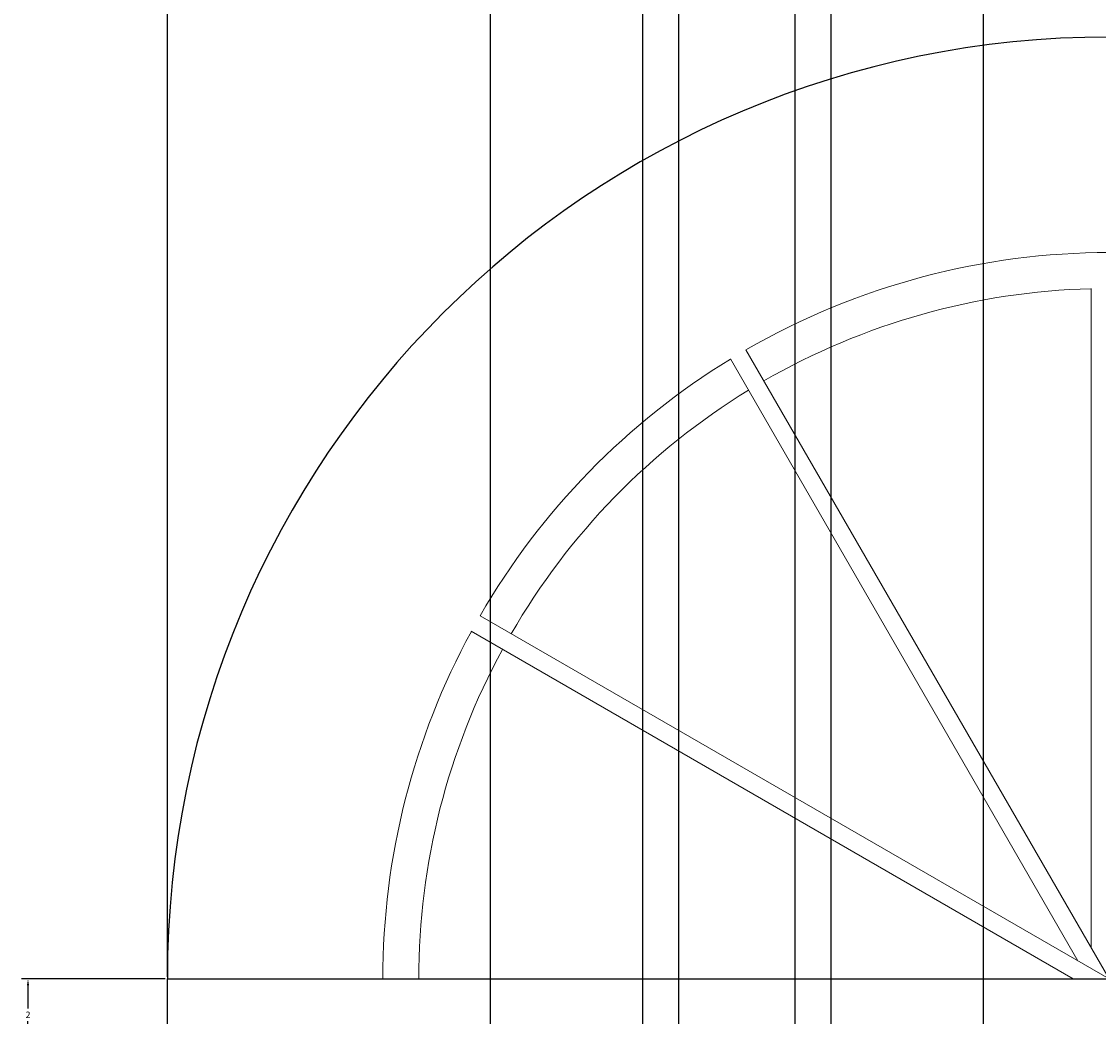
# Model space of a CAD drawing. Units: inches. Extents: x 12532.3 to 12594.9, y 6967.5 to 7063.
# Tile 6 of 9: x 12532.4 to 12562.4, y 7019.9 to 7047.6. Entities that reach past the tile are written whole.
import ezdxf

# ---------------------------------------------------------------- set-up
doc = ezdxf.new("R2010")
doc.units = ezdxf.units.IN
doc.header["$MEASUREMENT"] = 0
doc.header["$PDMODE"] = 98
for name, color, linetype, lineweight in [('A-ANNO-DIMS', 2, 'Continuous', 18), ('A-DOOR', 4, 'Continuous', 25), ('A-GLAZ', 3, 'Continuous', 18)]:
    doc.layers.add(name, color=color, linetype=linetype, lineweight=lineweight)
doc.styles.get("Standard").update_dxf_attribs({"font": 'arial.ttf'})
doc.dimstyles.get("Standard").update_dxf_attribs({"dimtxt": 0.18, "dimasz": 0.18, "dimexe": 0.18, "dimexo": 0.0625, "dimgap": 0.09, "dimtad": 0, "dimtih": 1, "dimtoh": 1, "dimdec": 4, "dimzin": 0, "dimdsep": 46, "dimtxsty": 'Standard', "dimcen": 0.09, "dimadec": 0, "dimazin": 0, "dimtfac": 1, "dimtdec": 4, "dimtofl": 0, "dimtmove": 0, "dimatfit": 3, "dimfxl": 1, "dimtolj": 1, "dimtzin": 0, "dimarcsym": 0})

# ---------------------------------------------------------------- blocks, each defined once
blk = doc.blocks.new('*D31')
at = {"layer": 'A-ANNO-DIMS', "color": 0, "lineweight": -2, "transparency": 16777216}
for p, q in [((12536.45, 7020.991), (12536.45, 7051.211)), ((12588.894, 7020.991), (12588.894, 7051.211)), ((12536.63, 7051.031), (12562.279, 7051.031)), ((12588.714, 7051.031), (12563.065, 7051.031))]:
    blk.add_line(p, q, dxfattribs=at)
at = {"layer": 'A-ANNO-DIMS', "color": 0, "transparency": 16777216}
for points in [[(12536.63, 7051.061), (12536.63, 7051.001), (12536.45, 7051.031)], [(12588.714, 7051.061), (12588.714, 7051.001), (12588.894, 7051.031)]]:
    blk.add_solid(points, dxfattribs=at)
at = {"layer": 'Defpoints', "color": 0, "transparency": 16777216}
for p in [(12588.894, 7051.031), (12536.45, 7020.929), (12588.894, 7020.929)]:
    blk.add_point(p, dxfattribs=at)
at = {"layer": 'A-ANNO-DIMS', "color": 0, "transparency": 16777216, "insert": (12562.672, 7051.031), "char_height": 0.18, "attachment_point": 5}
blk.add_mtext('\\A1;52.44', dxfattribs=at)
blk = doc.blocks.new('*D45')
at = {"layer": 'A-ANNO-DIMS', "color": 0, "lineweight": -2, "transparency": 16777216}
for p, q in [((12536.388, 7020.929), (12532.39, 7020.929)), ((12532.57, 7020.749), (12532.57, 7020.109)), ((12532.57, 7019.109), (12532.57, 7019.748)), ((12542.388, 7018.929), (12532.39, 7018.929))]:
    blk.add_line(p, q, dxfattribs=at)
at = {"layer": 'A-ANNO-DIMS', "color": 0, "transparency": 16777216}
for points in [[(12532.54, 7020.749), (12532.6, 7020.749), (12532.57, 7020.929)], [(12532.54, 7019.109), (12532.6, 7019.109), (12532.57, 7018.929)]]:
    blk.add_solid(points, dxfattribs=at)
at = {"layer": 'Defpoints', "color": 0, "transparency": 16777216}
for p in [(12532.57, 7020.929), (12536.45, 7020.929), (12542.45, 7018.929)]:
    blk.add_point(p, dxfattribs=at)
at = {"layer": 'A-ANNO-DIMS', "color": 0, "transparency": 16777216, "insert": (12532.57, 7019.929), "char_height": 0.18, "attachment_point": 5}
blk.add_mtext('\\A1;2', dxfattribs=at)
blk = doc.blocks.new('*D46')
at = {"layer": 'A-ANNO-DIMS', "color": 0, "lineweight": -2, "transparency": 16777216}
for p, q in [((12545.45, 7015.991), (12545.45, 7051.211)), ((12549.691, 7015.991), (12549.691, 7051.211)), ((12545.63, 7051.031), (12547.191, 7051.031)), ((12549.511, 7051.031), (12547.95, 7051.031))]:
    blk.add_line(p, q, dxfattribs=at)
at = {"layer": 'A-ANNO-DIMS', "color": 0, "transparency": 16777216}
for points in [[(12545.63, 7051.061), (12545.63, 7051.001), (12545.45, 7051.031)], [(12549.511, 7051.061), (12549.511, 7051.001), (12549.691, 7051.031)]]:
    blk.add_solid(points, dxfattribs=at)
at = {"layer": 'Defpoints', "color": 0, "transparency": 16777216}
for p in [(12549.691, 7051.031), (12545.45, 7015.929), (12549.691, 7015.929)]:
    blk.add_point(p, dxfattribs=at)
at = {"layer": 'A-ANNO-DIMS', "color": 0, "transparency": 16777216, "insert": (12547.57, 7051.031), "char_height": 0.18, "attachment_point": 5}
blk.add_mtext('\\A1;4.241', dxfattribs=at)
blk = doc.blocks.new('*D47')
at = {"layer": 'A-ANNO-DIMS', "color": 0, "lineweight": -2, "transparency": 16777216}
for p, q in [((12549.691, 7015.991), (12549.691, 7051.211)), ((12550.691, 7015.991), (12550.691, 7051.211)), ((12549.871, 7051.031), (12550.068, 7051.031)), ((12550.511, 7051.031), (12550.314, 7051.031))]:
    blk.add_line(p, q, dxfattribs=at)
at = {"layer": 'A-ANNO-DIMS', "color": 0, "transparency": 16777216}
for points in [[(12549.871, 7051.061), (12549.871, 7051.001), (12549.691, 7051.031)], [(12550.511, 7051.061), (12550.511, 7051.001), (12550.691, 7051.031)]]:
    blk.add_solid(points, dxfattribs=at)
at = {"layer": 'Defpoints', "color": 0, "transparency": 16777216}
for p in [(12550.691, 7051.031), (12549.691, 7015.929), (12550.691, 7015.929)]:
    blk.add_point(p, dxfattribs=at)
at = {"layer": 'A-ANNO-DIMS', "color": 0, "transparency": 16777216, "insert": (12550.191, 7051.031), "char_height": 0.18, "attachment_point": 5}
blk.add_mtext('\\A1;1', dxfattribs=at)
blk = doc.blocks.new('*D48')
at = {"layer": 'A-ANNO-DIMS', "color": 0, "lineweight": -2, "transparency": 16777216}
for p, q in [((12550.691, 7015.991), (12550.691, 7051.211)), ((12553.931, 7015.991), (12553.931, 7051.211)), ((12550.871, 7051.031), (12551.988, 7051.031)), ((12553.751, 7051.031), (12552.634, 7051.031))]:
    blk.add_line(p, q, dxfattribs=at)
at = {"layer": 'A-ANNO-DIMS', "color": 0, "transparency": 16777216}
for points in [[(12550.871, 7051.061), (12550.871, 7051.001), (12550.691, 7051.031)], [(12553.751, 7051.061), (12553.751, 7051.001), (12553.931, 7051.031)]]:
    blk.add_solid(points, dxfattribs=at)
at = {"layer": 'Defpoints', "color": 0, "transparency": 16777216}
for p in [(12553.931, 7051.031), (12550.691, 7015.929), (12553.931, 7015.929)]:
    blk.add_point(p, dxfattribs=at)
at = {"layer": 'A-ANNO-DIMS', "color": 0, "transparency": 16777216, "insert": (12552.311, 7051.031), "char_height": 0.18, "attachment_point": 5}
blk.add_mtext('\\A1;3.24', dxfattribs=at)
blk = doc.blocks.new('*D49')
at = {"layer": 'A-ANNO-DIMS', "color": 0, "lineweight": -2, "transparency": 16777216}
for p, q in [((12553.931, 7015.991), (12553.931, 7051.211)), ((12554.931, 7015.991), (12554.931, 7051.211)), ((12554.111, 7051.031), (12554.308, 7051.031)), ((12554.751, 7051.031), (12554.555, 7051.031))]:
    blk.add_line(p, q, dxfattribs=at)
at = {"layer": 'A-ANNO-DIMS', "color": 0, "transparency": 16777216}
for points in [[(12554.111, 7051.061), (12554.111, 7051.001), (12553.931, 7051.031)], [(12554.751, 7051.061), (12554.751, 7051.001), (12554.931, 7051.031)]]:
    blk.add_solid(points, dxfattribs=at)
at = {"layer": 'Defpoints', "color": 0, "transparency": 16777216}
for p in [(12554.931, 7051.031), (12553.931, 7015.929), (12554.931, 7015.929)]:
    blk.add_point(p, dxfattribs=at)
at = {"layer": 'A-ANNO-DIMS', "color": 0, "transparency": 16777216, "insert": (12554.431, 7051.031), "char_height": 0.18, "attachment_point": 5}
blk.add_mtext('\\A1;1', dxfattribs=at)
blk = doc.blocks.new('*D50')
at = {"layer": 'A-ANNO-DIMS', "color": 0, "lineweight": -2, "transparency": 16777216}
for p, q in [((12554.931, 7015.991), (12554.931, 7051.211)), ((12559.172, 7015.991), (12559.172, 7051.211)), ((12555.111, 7051.031), (12556.672, 7051.031)), ((12558.992, 7051.031), (12557.432, 7051.031))]:
    blk.add_line(p, q, dxfattribs=at)
at = {"layer": 'A-ANNO-DIMS', "color": 0, "transparency": 16777216}
for points in [[(12555.111, 7051.061), (12555.111, 7051.001), (12554.931, 7051.031)], [(12558.992, 7051.061), (12558.992, 7051.001), (12559.172, 7051.031)]]:
    blk.add_solid(points, dxfattribs=at)
at = {"layer": 'Defpoints', "color": 0, "transparency": 16777216}
for p in [(12559.172, 7051.031), (12554.931, 7015.929), (12559.172, 7015.929)]:
    blk.add_point(p, dxfattribs=at)
at = {"layer": 'A-ANNO-DIMS', "color": 0, "transparency": 16777216, "insert": (12557.052, 7051.031), "char_height": 0.18, "attachment_point": 5}
blk.add_mtext('\\A1;4.241', dxfattribs=at)
blk = doc.blocks.new('*D62')
at = {"layer": 'A-ANNO-DIMS', "color": 0, "lineweight": -2, "transparency": 16777216}
for p, q in [((12562.489, 7062.884), (12562.669, 7062.884)), ((12562.669, 7062.884), (12562.67, 7047.331)), ((12562.582, 7020.929), (12562.762, 7020.929)), ((12562.672, 7020.839), (12562.672, 7021.019))]:
    blk.add_line(p, q, dxfattribs=at)
at = {"layer": 'A-ANNO-DIMS', "color": 0, "transparency": 16777216}
blk.add_solid([(12562.7, 7047.331), (12562.64, 7047.331), (12562.67, 7047.151)], dxfattribs=at)
at = {"layer": 'Defpoints', "color": 0, "transparency": 16777216}
for p in [(12562.67, 7047.151), (12562.672, 7020.929)]:
    blk.add_point(p, dxfattribs=at)
at = {"layer": 'A-ANNO-DIMS', "color": 0, "transparency": 16777216, "insert": (12562.01, 7062.884), "char_height": 0.18, "attachment_point": 5}
blk.add_mtext('\\A1;R26.22', dxfattribs=at)

msp = doc.modelspace()

# ---------------------------------------------------------------- linework, layer by layer
at = {"layer": 'A-DOOR'}
msp.add_lwpolyline([(12536.4501, 7020.9287), (12588.894, 7020.9287), (12588.894, 6971.5968), (12536.4501, 6971.5968)], close=True, dxfattribs=at)
msp.add_arc((12562.6721, 7020.9287), 26.2219, 0, 180, dxfattribs=at)
at = {"layer": 'A-GLAZ'}
for p, q in [((12562.1721, 7021.7947), (12562.1721, 7040.1506)), ((12562.6721, 7020.9287), (12552.5611, 7038.4414)), ((12561.806, 7021.4287), (12552.1281, 7038.1914)), ((12562.6721, 7020.9287), (12545.1594, 7031.0397)), ((12561.6721, 7020.9287), (12544.9094, 7030.6067))]:
    msp.add_line(p, q, dxfattribs=at)
for radius, start, end in [(20.2219, 60, 120), (19.2219, 91.49054, 120), (20.2219, 121.41682, 150), (19.2219, 121.49054, 150), (20.2219, 151.41682, 180), (19.2219, 151.49054, 180)]:
    msp.add_arc((12562.6721, 7020.9287), radius, start, end, dxfattribs=at)

# ---------------------------------------------------------------- dimensions: what is measured, and where the dimension line sits
at = {"layer": 'A-ANNO-DIMS'}
dim = msp.add_radius_dim(center=(12562.6721, 7020.9287), mpoint=(12562.67, 7047.1506), dimstyle='Standard', override={"dimdec": 2, "dimlfac": 1, "dimrnd": 0, "dimzin": 0, "dimdsep": 46, "dimlunit": 2}, dxfattribs=at)
dim.commit()
dim.dimension.update_dxf_attribs({"geometry": '*D62', "text_midpoint": (12562.0098, 7062.8838), "dimtype": 164})
for base, p1, p2, override, picture, middle in [((12588.894, 7051.0306), (12536.4501, 7020.9287), (12588.894, 7020.9287), {"dimdec": 2, "dimlfac": 1, "dimrnd": 0, "dimzin": 0, "dimdsep": 46, "dimlunit": 2}, '*D31', (12562.6721, 7051.0306)), ((12549.6908, 7051.0306), (12545.4501, 7015.9287), (12549.6908, 7015.9287), {"dimdec": 3, "dimlfac": 1, "dimrnd": 0, "dimzin": 0, "dimdsep": 46, "dimlunit": 2}, '*D46', (12547.5705, 7051.0306)), ((12550.6908, 7051.0306), (12549.6908, 7015.9287), (12550.6908, 7015.9287), {"dimdec": 0, "dimlfac": 1, "dimrnd": 0, "dimzin": 0, "dimdsep": 46, "dimlunit": 2}, '*D47', (12550.1908, 7051.0306)), ((12553.9314, 7051.0306), (12550.6908, 7015.9287), (12553.9314, 7015.9287), {"dimdec": 2, "dimlfac": 1, "dimrnd": 0, "dimzin": 0, "dimdsep": 46, "dimlunit": 2}, '*D48', (12552.3111, 7051.0306)), ((12554.9314, 7051.0306), (12553.9314, 7015.9287), (12554.9314, 7015.9287), {"dimdec": 0, "dimlfac": 1, "dimrnd": 0, "dimzin": 0, "dimdsep": 46, "dimlunit": 2}, '*D49', (12554.4314, 7051.0306)), ((12559.1721, 7051.0306), (12554.9314, 7015.9287), (12559.1721, 7015.9287), {"dimdec": 3, "dimlfac": 1, "dimrnd": 0, "dimzin": 0, "dimdsep": 46, "dimlunit": 2}, '*D50', (12557.0518, 7051.0306))]:
    dim = msp.add_linear_dim(base=base, p1=p1, p2=p2, dimstyle='Standard', override=override, dxfattribs=at)
    dim.commit()
    dim.dimension.update_dxf_attribs({"geometry": picture, "text_midpoint": middle})
dim = msp.add_linear_dim(base=(12532.5701, 7020.9287), p1=(12542.4501, 7018.9287), p2=(12536.4501, 7020.9287), angle=90, dimstyle='Standard', override={"dimdec": 0, "dimlfac": 1, "dimrnd": 0, "dimzin": 0, "dimdsep": 46, "dimlunit": 2}, dxfattribs=at)
dim.commit()
dim.dimension.update_dxf_attribs({"geometry": '*D45', "text_midpoint": (12532.5701, 7019.9287)})

doc.saveas('drawing.dxf')
